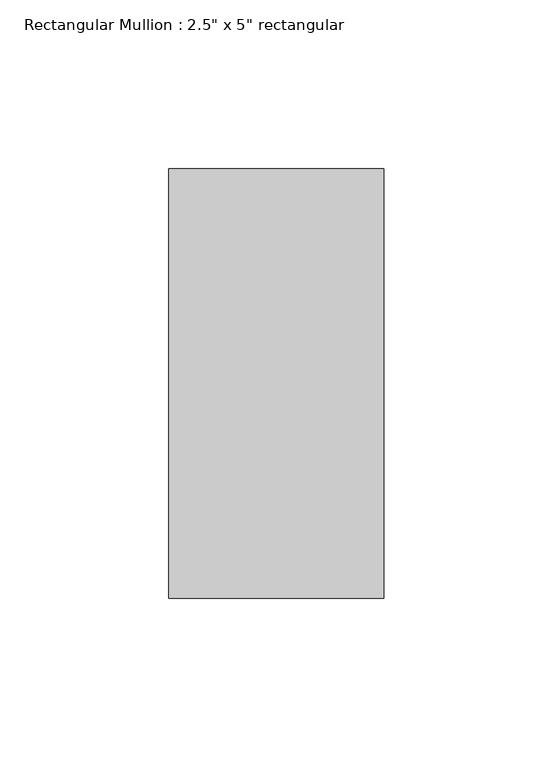
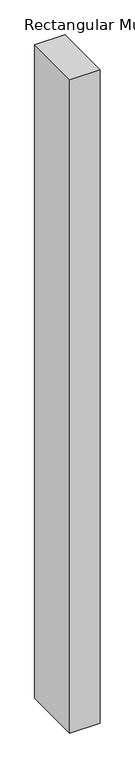
"""IFC4 building model written with IfcOpenShell, lengths in millimetres: member geometry."""

from ifc_helpers import new_model, si_unit, frame, origin, place, context, project, spatial, polyline, outline, extrude, source, transform, mapped, element, save


def member_e55e8fcb(model_context):
    return source(origin(), model_context, "Body", "SweptSolid", [
        extrude(outline(polyline([(0.0, 63.5), (0.0, -63.5), (-63.5, -63.5), (-63.5, 63.5), (0.0, 63.5)])), frame((0.0, 0.0, -1447.0507887), z_axis=(0.0, 0.0, 1.0), x_axis=(1.0, 0.0, 0.0)), (0.0, 0.0, 1.0), 1447.0507887),
    ])


if __name__ == "__main__":
    model = new_model("IFC4")
    model_context = context("Model", 3, world=origin())
    ifc_project = project(units=[si_unit("LENGTHUNIT", "METRE", prefix="MILLI")], contexts=[model_context])
    site = spatial("IfcSite", under=ifc_project)
    building = spatial("IfcBuilding", under=site)
    placement = place(None, origin())
    member_shape = member_e55e8fcb(model_context)
    element("IfcMember", 1, ObjectType="Rectangular Mullion : 2.5\" x 5\" rectangular", at=placement, inside=building, context=model_context, shape_type="MappedRepresentation", body=[
        mapped(member_shape, transform((0.0, 0.0, 0.0), x_axis=(1.0, 0.0, 0.0), y_axis=(0.0, 1.0, 0.0), z_axis=(0.0, 0.0, 1.0))),
    ])
    save(model, "model.ifc")

# Revit data of these elements
# Type "Rectangular Mullion : 2.5\" x 5\" rectangular"
#   built-in parameter 1007304 = 0.416667 (stored number, unit not read)
#   built-in parameter 1007301 = 0.104167 (stored number, unit not read)
#   built-in parameter 1007300 = 0.104167 (stored number, unit not read)
# Element 1 (IfcMember, "Rectangular Mullion : 2.5\" x 5\" rectangular")
#   Materials on its faces: "Aluminum"
# Materials
#   "Aluminum": class "Metal", colour RGB 247 247 247, transparency 0, Description = "Aluminum 6061", Cost = 0
